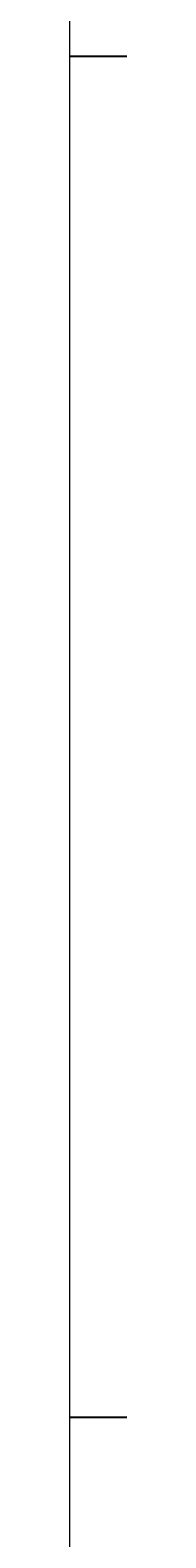
# Model space of a CAD drawing. Units: inches. Extents: x 35362 to 73946, y 43607 to 67532.
# Tile 44 of 134: x 48377 to 48389, y 46091 to 46564. Entities that reach past the tile are written whole.
import ezdxf

# ---------------------------------------------------------------- set-up
doc = ezdxf.new("R2010")
doc.units = ezdxf.units.IN
doc.header["$MEASUREMENT"] = 0
doc.layers.add('A-ANNO-DIMS', color=2, linetype='Continuous', lineweight=18)
doc.styles.get("Standard").update_dxf_attribs({"font": 'arial.ttf'})
doc.dimstyles.get("Standard").update_dxf_attribs({"dimtxt": 0.18, "dimasz": 0.18, "dimexe": 0.18, "dimexo": 0.0625, "dimgap": 0.09, "dimtad": 0, "dimtih": 1, "dimtoh": 1, "dimdec": 4, "dimzin": 0, "dimdsep": 46, "dimtxsty": 'Standard', "dimcen": 0.09, "dimadec": 0, "dimazin": 0, "dimtfac": 1, "dimtdec": 4, "dimtofl": 0, "dimtmove": 0, "dimatfit": 3, "dimfxl": 1, "dimtolj": 1, "dimtzin": 0, "dimarcsym": 0})

# ---------------------------------------------------------------- blocks, each defined once
blk = doc.blocks.new('*D5')
at = {"layer": 'A-ANNO-DIMS', "color": 0, "lineweight": -2, "transparency": 16777216}
for p, q in [((37121.95, 46919.32), (37121.95, 43606.68)), ((69871.5, 45449.83), (69871.5, 43606.68)), ((37122.13, 43606.86), (53496.29, 43606.86)), ((69871.32, 43606.86), (53497.15, 43606.86))]:
    blk.add_line(p, q, dxfattribs=at)
at = {"layer": 'A-ANNO-DIMS', "color": 0, "transparency": 16777216}
for points in [[(37122.13, 43606.89), (37122.13, 43606.83), (37121.95, 43606.86)], [(69871.32, 43606.89), (69871.32, 43606.83), (69871.5, 43606.86)]]:
    blk.add_solid(points, dxfattribs=at)
at = {"layer": 'Defpoints', "color": 0, "transparency": 16777216}
for p in [(37121.95, 46919.38), (69871.5, 45449.89), (69871.5, 43606.86)]:
    blk.add_point(p, dxfattribs=at)
at = {"layer": 'A-ANNO-DIMS', "color": 0, "transparency": 16777216, "insert": (53496.72, 43606.86), "char_height": 0.18, "attachment_point": 5}
blk.add_mtext('\\A1;32750', dxfattribs=at)
blk = doc.blocks.new('*D11')
at = {"layer": 'A-ANNO-DIMS', "color": 0, "lineweight": -2, "transparency": 16777216}
for p, q in [((47978.66, 56028.77), (47978.66, 43606.68)), ((53109.76, 56028.77), (53109.76, 43606.68)), ((47978.84, 43606.86), (50543.87, 43606.86)), ((53109.58, 43606.86), (50544.55, 43606.86))]:
    blk.add_line(p, q, dxfattribs=at)
at = {"layer": 'A-ANNO-DIMS', "color": 0, "transparency": 16777216}
for points in [[(47978.84, 43606.89), (47978.84, 43606.83), (47978.66, 43606.86)], [(53109.58, 43606.89), (53109.58, 43606.83), (53109.76, 43606.86)]]:
    blk.add_solid(points, dxfattribs=at)
at = {"layer": 'Defpoints', "color": 0, "transparency": 16777216}
for p in [(47978.66, 56028.84), (53109.76, 56028.84), (53109.76, 43606.86)]:
    blk.add_point(p, dxfattribs=at)
at = {"layer": 'A-ANNO-DIMS', "color": 0, "transparency": 16777216, "insert": (50544.21, 43606.86), "char_height": 0.18, "attachment_point": 5}
blk.add_mtext('\\A1;5131', dxfattribs=at)
blk = doc.blocks.new('*D13')
at = {"layer": 'A-ANNO-DIMS', "color": 0, "lineweight": -2, "transparency": 16777216}
for p, q in [((48373.49, 51694.02), (48373.49, 43606.68)), ((51029.04, 51694.02), (51029.04, 43606.68)), ((48373.67, 43606.86), (49700.8, 43606.86)), ((51028.86, 43606.86), (49701.73, 43606.86))]:
    blk.add_line(p, q, dxfattribs=at)
at = {"layer": 'A-ANNO-DIMS', "color": 0, "transparency": 16777216}
for points in [[(48373.67, 43606.89), (48373.67, 43606.83), (48373.49, 43606.86)], [(51028.86, 43606.89), (51028.86, 43606.83), (51029.04, 43606.86)]]:
    blk.add_solid(points, dxfattribs=at)
at = {"layer": 'Defpoints', "color": 0, "transparency": 16777216}
for p in [(48373.49, 51694.09), (51029.04, 51694.09), (51029.04, 43606.86)]:
    blk.add_point(p, dxfattribs=at)
at = {"layer": 'A-ANNO-DIMS', "color": 0, "transparency": 16777216, "insert": (49701.27, 43606.86), "char_height": 0.18, "attachment_point": 5}
blk.add_mtext('\\A1;2655.6', dxfattribs=at)
blk = doc.blocks.new('*D67')
at = {"layer": 'A-ANNO-DIMS', "color": 0, "lineweight": -2, "transparency": 16777216}
for p, q in [((56873.54, 53351.53), (35361.77, 53351.53)), ((35361.95, 53351.35), (35361.95, 49400.89)), ((35361.95, 45450.07), (35361.95, 49400.53)), ((53793.58, 45449.89), (35361.77, 45449.89))]:
    blk.add_line(p, q, dxfattribs=at)
at = {"layer": 'A-ANNO-DIMS', "color": 0, "transparency": 16777216}
for points in [[(35361.92, 53351.35), (35361.98, 53351.35), (35361.95, 53351.53)], [(35361.92, 45450.07), (35361.98, 45450.07), (35361.95, 45449.89)]]:
    blk.add_solid(points, dxfattribs=at)
at = {"layer": 'Defpoints', "color": 0, "transparency": 16777216}
for p in [(35361.95, 53351.53), (56873.6, 53351.53), (53793.64, 45449.89)]:
    blk.add_point(p, dxfattribs=at)
at = {"layer": 'A-ANNO-DIMS', "color": 0, "transparency": 16777216, "insert": (35361.95, 49400.71), "char_height": 0.18, "attachment_point": 5}
blk.add_mtext('\\A1;7901.6', dxfattribs=at)
blk = doc.blocks.new('*D76')
at = {"layer": 'A-ANNO-DIMS', "color": 0, "lineweight": -2, "transparency": 16777216}
for p, q in [((54052.84, 46555.29), (35361.77, 46555.29)), ((35361.95, 46555.11), (35361.95, 46342.27)), ((35361.95, 46129.06), (35361.95, 46341.9)), ((53793.58, 46128.88), (35361.77, 46128.88))]:
    blk.add_line(p, q, dxfattribs=at)
at = {"layer": 'A-ANNO-DIMS', "color": 0, "transparency": 16777216}
for points in [[(35361.92, 46555.11), (35361.98, 46555.11), (35361.95, 46555.29)], [(35361.92, 46129.06), (35361.98, 46129.06), (35361.95, 46128.88)]]:
    blk.add_solid(points, dxfattribs=at)
at = {"layer": 'Defpoints', "color": 0, "transparency": 16777216}
for p in [(35361.95, 46555.29), (54052.9, 46555.29), (53793.64, 46128.88)]:
    blk.add_point(p, dxfattribs=at)
at = {"layer": 'A-ANNO-DIMS', "color": 0, "transparency": 16777216, "insert": (35361.95, 46342.09), "char_height": 0.18, "attachment_point": 5}
blk.add_mtext('\\A1;426.4', dxfattribs=at)
blk = doc.blocks.new('*D90')
at = {"layer": 'A-ANNO-DIMS', "color": 0, "lineweight": -2, "transparency": 16777216}
for p, q in [((53707.72, 47291.29), (35361.77, 47291.29)), ((35361.95, 47291.11), (35361.95, 46710.26)), ((35361.95, 46129.06), (35361.95, 46709.9)), ((53793.58, 46128.88), (35361.77, 46128.88))]:
    blk.add_line(p, q, dxfattribs=at)
at = {"layer": 'A-ANNO-DIMS', "color": 0, "transparency": 16777216}
for points in [[(35361.92, 47291.11), (35361.98, 47291.11), (35361.95, 47291.29)], [(35361.92, 46129.06), (35361.98, 46129.06), (35361.95, 46128.88)]]:
    blk.add_solid(points, dxfattribs=at)
at = {"layer": 'Defpoints', "color": 0, "transparency": 16777216}
for p in [(53707.78, 47291.29), (35361.95, 46128.88), (53793.64, 46128.88)]:
    blk.add_point(p, dxfattribs=at)
at = {"layer": 'A-ANNO-DIMS', "color": 0, "transparency": 16777216, "insert": (35361.95, 46710.08), "char_height": 0.18, "attachment_point": 5}
blk.add_mtext('\\A1;1162.4', dxfattribs=at)

msp = doc.modelspace()

# ---------------------------------------------------------------- dimensions: what is measured, and where the dimension line sits
at = {"layer": 'A-ANNO-DIMS'}
for base, p1, p2, override, picture, middle in [((53109.76, 43606.859), (47978.665, 56028.836), (53109.76, 56028.836), {"dimdec": 0, "dimlfac": 1, "dimrnd": 0, "dimzin": 0, "dimdsep": 46, "dimlunit": 2}, '*D11', (50544.212, 43606.859)), ((51029.043, 43606.859), (48373.492, 51694.087), (51029.043, 51694.087), {"dimdec": 1, "dimlfac": 1, "dimrnd": 0, "dimzin": 0, "dimdsep": 46, "dimlunit": 2}, '*D13', (49701.267, 43606.859)), ((69871.496, 43606.859), (37121.949, 46919.381), (69871.496, 45449.894), {"dimdec": 0, "dimlfac": 1, "dimrnd": 0, "dimzin": 0, "dimdsep": 46, "dimlunit": 2}, '*D5', (53496.723, 43606.859))]:
    dim = msp.add_linear_dim(base=base, p1=p1, p2=p2, dimstyle='Standard', override=override, dxfattribs=at)
    dim.commit()
    dim.dimension.update_dxf_attribs({"geometry": picture, "text_midpoint": middle})
for base, p1, p2, picture, middle in [((35361.949, 53351.529), (53793.638, 45449.894), (56873.602, 53351.529), '*D67', (35361.949, 49400.712)), ((35361.949, 46128.878), (53707.781, 47291.285), (53793.638, 46128.878), '*D90', (35361.949, 46710.081)), ((35361.949, 46555.293), (53793.638, 46128.878), (54052.899, 46555.293), '*D76', (35361.949, 46342.086))]:
    dim = msp.add_linear_dim(base=base, p1=p1, p2=p2, angle=90, dimstyle='Standard', override={"dimdec": 1, "dimlfac": 1, "dimrnd": 0, "dimzin": 0, "dimdsep": 46, "dimlunit": 2}, dxfattribs=at)
    dim.commit()
    dim.dimension.update_dxf_attribs({"geometry": picture, "text_midpoint": middle})

doc.saveas('drawing.dxf')
